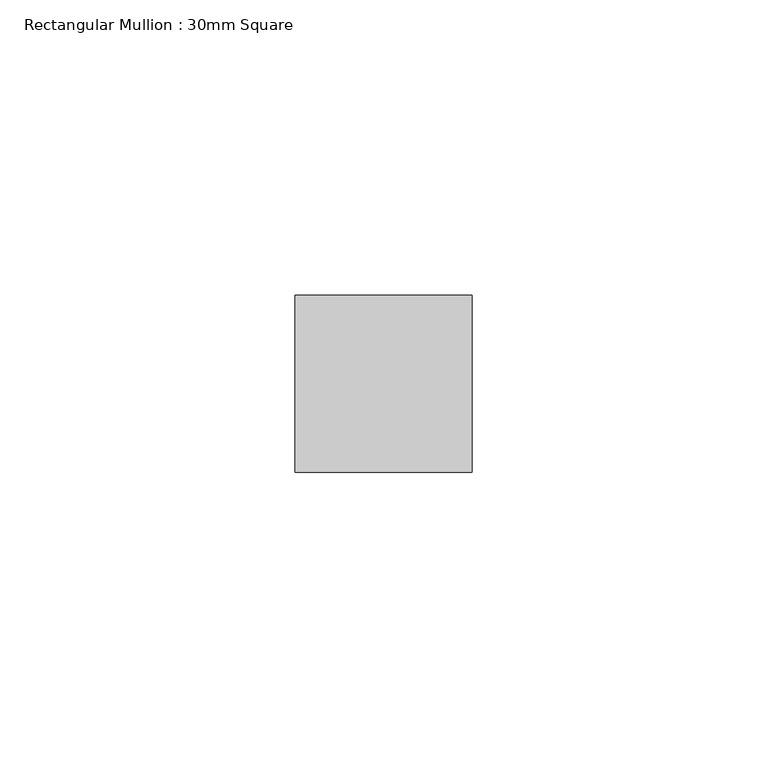
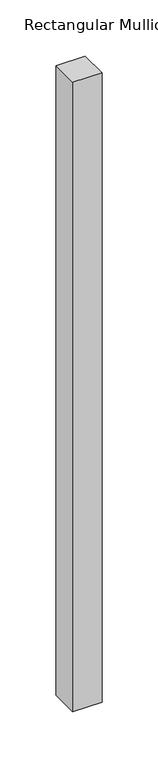
"""IFC4 building model written with IfcOpenShell, lengths in millimetres: member geometry, Rectangular Mullion : 30mm Square."""

from ifc_helpers import new_model, si_unit, frame, origin, place, context, project, spatial, polyline, outline, extrude, source, transform, mapped, element, save


def rectangular_mullion_30mm_square_88df2287(model_context):
    return source(origin(), model_context, "Body", "SweptSolid", [
        extrude(outline(polyline([(0.0, 15.0), (0.0, -15.0), (-30.0, -15.0), (-30.0, 15.0), (0.0, 15.0)])), frame((0.0, 0.0, -685.0), z_axis=(0.0, 0.0, 1.0), x_axis=(1.0, 0.0, 0.0)), (0.0, 0.0, 1.0), 685.0),
    ])


if __name__ == "__main__":
    model = new_model("IFC4")
    model_context = context("Model", 3, world=origin())
    ifc_project = project(units=[si_unit("LENGTHUNIT", "METRE", prefix="MILLI")], contexts=[model_context])
    site = spatial("IfcSite", under=ifc_project)
    building = spatial("IfcBuilding", under=site)
    placement = place(None, origin())
    rectangular_mullion_30mm_square_shape = rectangular_mullion_30mm_square_88df2287(model_context)
    element("IfcMember", 1, ObjectType="Rectangular Mullion : 30mm Square", at=placement, inside=building, context=model_context, shape_type="MappedRepresentation", body=[
        mapped(rectangular_mullion_30mm_square_shape, transform((0.0, 0.0, 0.0), x_axis=(1.0, 0.0, 0.0), y_axis=(0.0, 1.0, 0.0), z_axis=(0.0, 0.0, 1.0))),
    ])
    save(model, "model.ifc")

# Revit data of these elements
# Type "Rectangular Mullion : 30mm Square"
#   built-in parameter 1007304 = 0.0984252 (stored number, unit not read)
#   built-in parameter 1007301 = 0.0492126 (stored number, unit not read)
#   built-in parameter 1007300 = 0.0492126 (stored number, unit not read)
# Element 1 (IfcMember, "Rectangular Mullion : 30mm Square")
#   Materials on its faces: "Aluminum"
# Materials
#   "Aluminum": class "Metal", colour RGB 244 244 244, transparency 0, Description = "Aluminum 6061", Cost = 0
